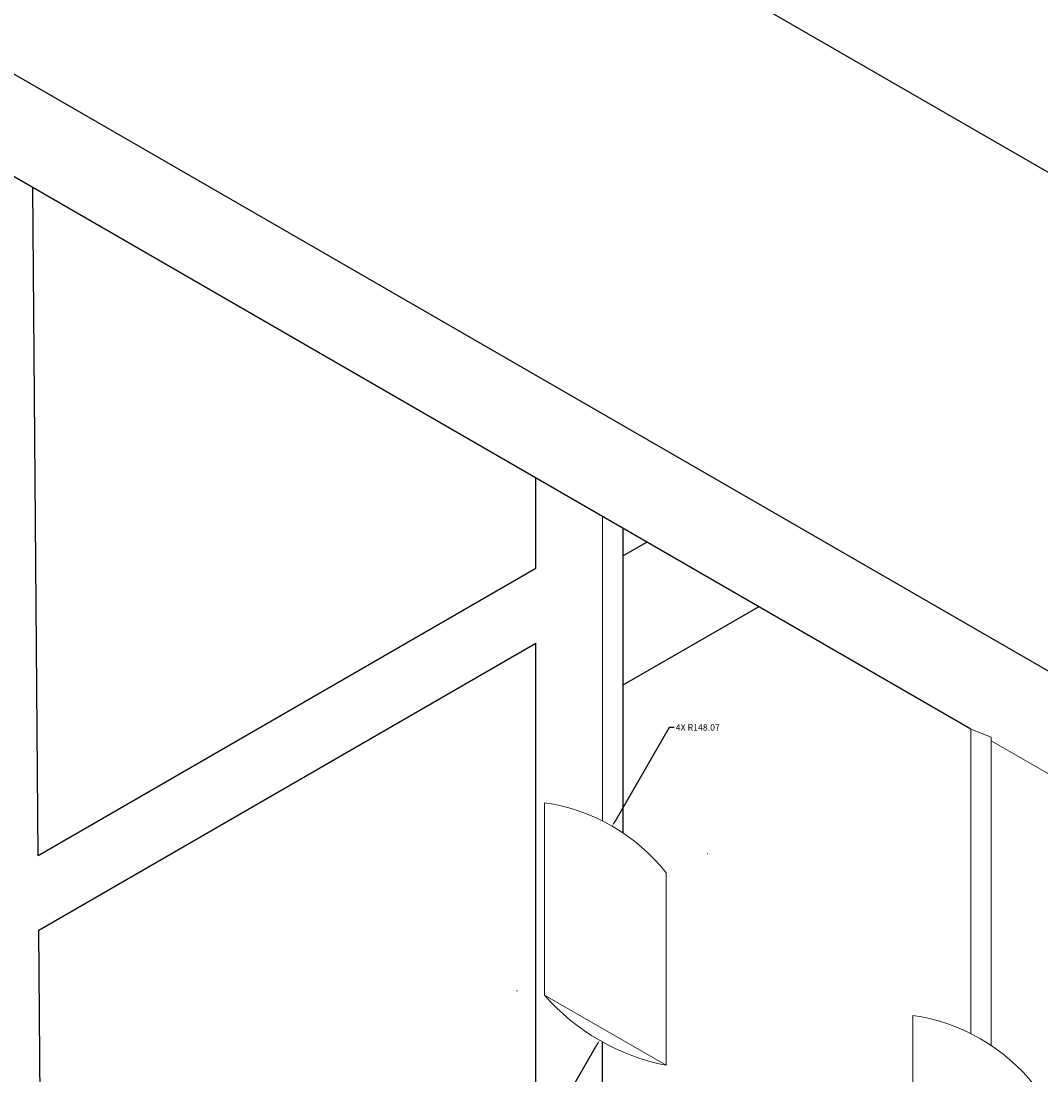
# Model space of a CAD drawing. Units: metres. Extents: x -2391 to 4922, y -635 to 4845.
# Tile 15 of 37: x -1981 to -1186, y 2190 to 3011. Entities that reach past the tile are written whole.
import ezdxf

# ---------------------------------------------------------------- set-up
doc = ezdxf.new("R2010")
doc.units = ezdxf.units.M
doc.header["$MEASUREMENT"] = 0
for name, color, linetype, lineweight in [('A-ANNO-DIMS', 2, 'Continuous', 18), ('A-EQPM', 9, 'Continuous', 18), ('A-FLOR-FIXT', 3, 'Continuous', 25)]:
    doc.layers.add(name, color=color, linetype=linetype, lineweight=lineweight)
doc.styles.get("Standard").update_dxf_attribs({"font": 'arial.ttf'})
doc.dimstyles.get("Standard").update_dxf_attribs({"dimtxt": 5, "dimasz": 4, "dimexe": 0.18, "dimexo": 0.0625, "dimgap": 0.09, "dimtad": 0, "dimtih": 1, "dimtoh": 1, "dimdec": 0, "dimzin": 0, "dimdsep": 46, "dimtxsty": 'Standard', "dimcen": 0.09, "dimadec": 0, "dimazin": 0, "dimtfac": 1, "dimtdec": 0, "dimtofl": 0, "dimtmove": 0, "dimatfit": 3, "dimfxl": 1, "dimtolj": 1, "dimtzin": 0, "dimarcsym": 0})

# ---------------------------------------------------------------- blocks, each defined once
blk = doc.blocks.new('UTENSIL-HANGING')
for p, q in [((0, 204.54), (0, 54.7)), ((94.74, 0), (94.74, 149.84)), ((0, 54.7), (94.74, 0))]:
    blk.add_line(p, q)
for centre, radius, start, end in [((-21.43, 58.03), 148.07, 38.32024, 81.67976), ((126.83, 164.98), 168.07, 221.00715, 258.99285)]:
    blk.add_arc(centre, radius, start, end)
blk = doc.blocks.new('*D8')
at = {"layer": 'A-ANNO-DIMS', "color": 0, "lineweight": -2, "transparency": 16777216}
for p, q in [((-2047.33, 3005.21), (-2047.33, -631.4)), ((4577.76, 2350.21), (4577.76, -631.4)), ((-2043.33, -631.22), (1257.62, -631.22)), ((4573.76, -631.22), (1272.8, -631.22))]:
    blk.add_line(p, q, dxfattribs=at)
at = {"layer": 'A-ANNO-DIMS', "color": 0, "transparency": 16777216}
for points in [[(-2043.33, -630.56), (-2043.33, -631.89), (-2047.33, -631.22)], [(4573.76, -630.56), (4573.76, -631.89), (4577.76, -631.22)]]:
    blk.add_solid(points, dxfattribs=at)
at = {"layer": 'Defpoints', "color": 0, "transparency": 16777216}
for p in [(-2047.33, 3005.28), (4577.76, 2350.28), (4577.76, -631.22)]:
    blk.add_point(p, dxfattribs=at)
at = {"layer": 'A-ANNO-DIMS', "color": 0, "transparency": 16777216, "insert": (1265.21, -631.22), "char_height": 5, "attachment_point": 5}
blk.add_mtext('\\A1;6625', dxfattribs=at)
blk = doc.blocks.new('*D9')
at = {"layer": 'A-ANNO-DIMS', "color": 0, "lineweight": -2, "transparency": 16777216}
for p, q in [((-2047.33, 3005.34), (-2047.33, 4841.96)), ((-2043.33, 4841.78), (-755.9, 4841.78)), ((546.74, 4841.78), (-740.69, 4841.78)), ((550.74, 4505.34), (550.74, 4841.96))]:
    blk.add_line(p, q, dxfattribs=at)
at = {"layer": 'A-ANNO-DIMS', "color": 0, "transparency": 16777216}
for points in [[(-2043.33, 4842.44), (-2043.33, 4841.11), (-2047.33, 4841.78)], [(546.74, 4842.44), (546.74, 4841.11), (550.74, 4841.78)]]:
    blk.add_solid(points, dxfattribs=at)
at = {"layer": 'Defpoints', "color": 0, "transparency": 16777216}
for p in [(550.74, 4841.78), (550.74, 4505.28), (-2047.33, 3005.28)]:
    blk.add_point(p, dxfattribs=at)
at = {"layer": 'A-ANNO-DIMS', "color": 0, "transparency": 16777216, "insert": (-748.3, 4841.78), "char_height": 5, "attachment_point": 5}
blk.add_mtext('\\A1;2598', dxfattribs=at)
blk = doc.blocks.new('*D10')
at = {"layer": 'A-ANNO-DIMS', "color": 0, "lineweight": -2, "transparency": 16777216}
for p, q in [((550.68, 4505.28), (-2384.01, 4505.28)), ((-2383.83, 4501.28), (-2383.83, 2107.92)), ((-2383.83, -290.72), (-2383.83, 2102.63)), ((-488.55, -294.72), (-2384.01, -294.72))]:
    blk.add_line(p, q, dxfattribs=at)
at = {"layer": 'A-ANNO-DIMS', "color": 0, "transparency": 16777216}
for points in [[(-2384.5, 4501.28), (-2383.17, 4501.28), (-2383.83, 4505.28)], [(-2384.5, -290.72), (-2383.17, -290.72), (-2383.83, -294.72)]]:
    blk.add_solid(points, dxfattribs=at)
at = {"layer": 'Defpoints', "color": 0, "transparency": 16777216}
for p in [(-2383.83, 4505.28), (550.74, 4505.28), (-488.49, -294.72)]:
    blk.add_point(p, dxfattribs=at)
at = {"layer": 'A-ANNO-DIMS', "color": 0, "transparency": 16777216, "insert": (-2383.83, 2105.28), "char_height": 5, "attachment_point": 5}
blk.add_mtext('\\A1;4800', dxfattribs=at)
blk = doc.blocks.new('*D41')
at = {"layer": 'A-ANNO-DIMS', "color": 0, "lineweight": -2, "transparency": 16777216}
for p, q in [((-2047.3, 3005.33), (-1878.99, 3296.85)), ((-1875.62, 3294.69), (-1104.24, 2849.34)), ((-323.7, 2398.69), (-1095.08, 2844.05)), ((-488.46, 2105.33), (-320.15, 2396.85))]:
    blk.add_line(p, q, dxfattribs=at)
at = {"layer": 'A-ANNO-DIMS', "color": 0, "transparency": 16777216}
for points in [[(-1875.29, 3295.27), (-1875.95, 3294.12), (-1879.08, 3296.69)], [(-323.37, 2399.27), (-324.04, 2398.12), (-320.24, 2396.69)]]:
    blk.add_solid(points, dxfattribs=at)
at = {"layer": 'Defpoints', "color": 0, "transparency": 16777216}
for p in [(-2047.33, 3005.28), (-320.24, 2396.69), (-488.49, 2105.28)]:
    blk.add_point(p, dxfattribs=at)
at = {"layer": 'A-ANNO-DIMS', "color": 0, "transparency": 16777216, "insert": (-1099.66, 2846.69), "char_height": 5, "attachment_point": 5}
blk.add_mtext('\\A1;1800', dxfattribs=at)
blk = doc.blocks.new('*D52')
at = {"layer": 'A-ANNO-DIMS', "color": 0, "lineweight": -2, "transparency": 16777216}
for p, q in [((-1445.98, 2362.64), (-1445.8, 2362.64)), ((-1445.89, 2362.55), (-1445.89, 2362.73)), ((-1580.35, 2129.76), (-1531.93, 2213.63)), ((-1584.35, 2129.76), (-1580.35, 2129.76))]:
    blk.add_line(p, q, dxfattribs=at)
at = {"layer": 'A-ANNO-DIMS', "color": 0, "transparency": 16777216}
blk.add_solid([(-1532.51, 2213.96), (-1531.35, 2213.29), (-1529.93, 2217.09)], dxfattribs=at)
at = {"layer": 'Defpoints', "color": 0, "transparency": 16777216}
for p in [(-1445.89, 2362.64), (-1529.93, 2217.09)]:
    blk.add_point(p, dxfattribs=at)
at = {"layer": 'A-ANNO-DIMS', "color": 0, "transparency": 16777216, "insert": (-1602.68, 2129.76), "char_height": 5, "attachment_point": 5}
blk.add_mtext('\\A1;4X R168.07', dxfattribs=at)
blk = doc.blocks.new('*D53')
at = {"layer": 'A-ANNO-DIMS', "color": 0, "lineweight": -2, "transparency": 16777216}
for p, q in [((-1475.7, 2460.86), (-1518.12, 2387.39)), ((-1471.7, 2460.86), (-1475.7, 2460.86)), ((-1594.24, 2255.69), (-1594.06, 2255.69)), ((-1594.15, 2255.6), (-1594.15, 2255.78))]:
    blk.add_line(p, q, dxfattribs=at)
at = {"layer": 'A-ANNO-DIMS', "color": 0, "transparency": 16777216}
blk.add_solid([(-1518.69, 2387.72), (-1517.54, 2387.05), (-1520.12, 2383.92)], dxfattribs=at)
at = {"layer": 'Defpoints', "color": 0, "transparency": 16777216}
for p in [(-1520.12, 2383.92), (-1594.15, 2255.69)]:
    blk.add_point(p, dxfattribs=at)
at = {"layer": 'A-ANNO-DIMS', "color": 0, "transparency": 16777216, "insert": (-1453.36, 2460.86), "char_height": 5, "attachment_point": 5}
blk.add_mtext('\\A1;4X R148.07', dxfattribs=at)

msp = doc.modelspace()

# ---------------------------------------------------------------- linework, layer by layer
at = {"layer": 'A-EQPM'}
for p, q in [((-1527.7191, 2625.2763), (-1527.7191, 2388.0202)), ((-1527.7191, 2388.0202), (-1527.7191, 2625.2763)), ((-1240.7842, 2459.6143), (-1224.8889, 2453.2326)), ((-1240.7842, 2459.6143), (-1240.7842, 2222.3583)), ((-1224.8889, 2453.2326), (-1224.8889, 2213.1002)), ((-968.1457, 2302.2064), (-1224.8889, 2450.4372))]:
    msp.add_line(p, q, dxfattribs=at)
at = {"layer": 'A-FLOR-FIXT'}
for p, q in [((-2047.3343, 3005.2763), (-488.4886, 2105.2763)), ((-1240.7842, 2459.6143), (-2047.3343, 2925.2763)), ((-1967.2581, 2361.1289), (-1971.3744, 2881.4208)), ((-1579.6432, 2584.9185), (-1579.6432, 2655.2547)), ((-1511.8238, 2616.0991), (-1511.8238, 2378.7621)), ((-1511.8238, 2594.4534), (-1493.0781, 2605.2763)), ((-1967.2581, 2361.1289), (-1579.6432, 2584.9185)), ((-1405.8159, 2554.8954), (-1511.8238, 2493.6917)), ((-1966.7983, 2303.0012), (-1579.6432, 2526.5253)), ((-1579.6432, 2182.6221), (-1579.6432, 2526.5253)), ((-1964.0899, 1960.6617), (-1966.7983, 2303.0012)), ((-1527.7191, 1805.2763), (-1527.7191, 2215.836))]:
    msp.add_line(p, q, dxfattribs=at)

# ---------------------------------------------------------------- block references
at = {"layer": 'A-EQPM'}
for p in [(-1572.724, 2197.663), (-1285.7891, 2032.0011)]:
    msp.add_blockref('UTENSIL-HANGING', p, dxfattribs=at)

# ---------------------------------------------------------------- dimensions: what is measured, and where the dimension line sits
at = {"layer": 'A-ANNO-DIMS'}
for base, p2, picture, middle in [((550.7419, 4841.7763), (550.7419, 4505.2763), '*D9', (-748.2962, 4841.7763)), ((4577.76, -631.2237), (4577.76, 2350.2763), '*D8', (1265.2128, -631.2237))]:
    dim = msp.add_linear_dim(base=base, p1=(-2047.3343, 3005.2763), p2=p2, dimstyle='Standard', override={"dimdec": 0, "dimlfac": 1, "dimrnd": 0, "dimzin": 0, "dimdsep": 46, "dimlunit": 2}, dxfattribs=at)
    dim.commit()
    dim.dimension.update_dxf_attribs({"geometry": picture, "text_midpoint": middle})
for base, p1, p2, angle, picture, middle in [((-2383.8343, 4505.2763), (-488.4886, -294.7237), (550.7419, 4505.2763), 90, '*D10', (-2383.8343, 2105.2763)), ((-320.2386, 2396.6938), (-2047.3343, 3005.2763), (-488.4886, 2105.2763), 330, '*D41', (-1099.6615, 2846.6938))]:
    dim = msp.add_linear_dim(base=base, p1=p1, p2=p2, angle=angle, dimstyle='Standard', override={"dimdec": 0, "dimlfac": 1, "dimrnd": 0, "dimzin": 0, "dimdsep": 46, "dimlunit": 2}, dxfattribs=at)
    dim.commit()
    dim.dimension.update_dxf_attribs({"geometry": picture, "text_midpoint": middle})
for center, mpoint, picture, middle in [((-1594.1502, 2255.6899), (-1520.1158, 2383.9214), '*D53', (-1453.3616, 2460.8603)), ((-1445.8912, 2362.6446), (-1529.9279, 2217.0891), '*D52', (-1602.6835, 2129.7559))]:
    dim = msp.add_radius_dim(center=center, mpoint=mpoint, text='4X <>', dimstyle='Standard', override={"dimdec": 2, "dimlfac": 1, "dimrnd": 0, "dimzin": 0, "dimdsep": 46, "dimlunit": 2}, dxfattribs=at)
    dim.commit()
    dim.dimension.update_dxf_attribs({"geometry": picture, "text_midpoint": middle, "dimtype": 164})

doc.saveas('drawing.dxf')
